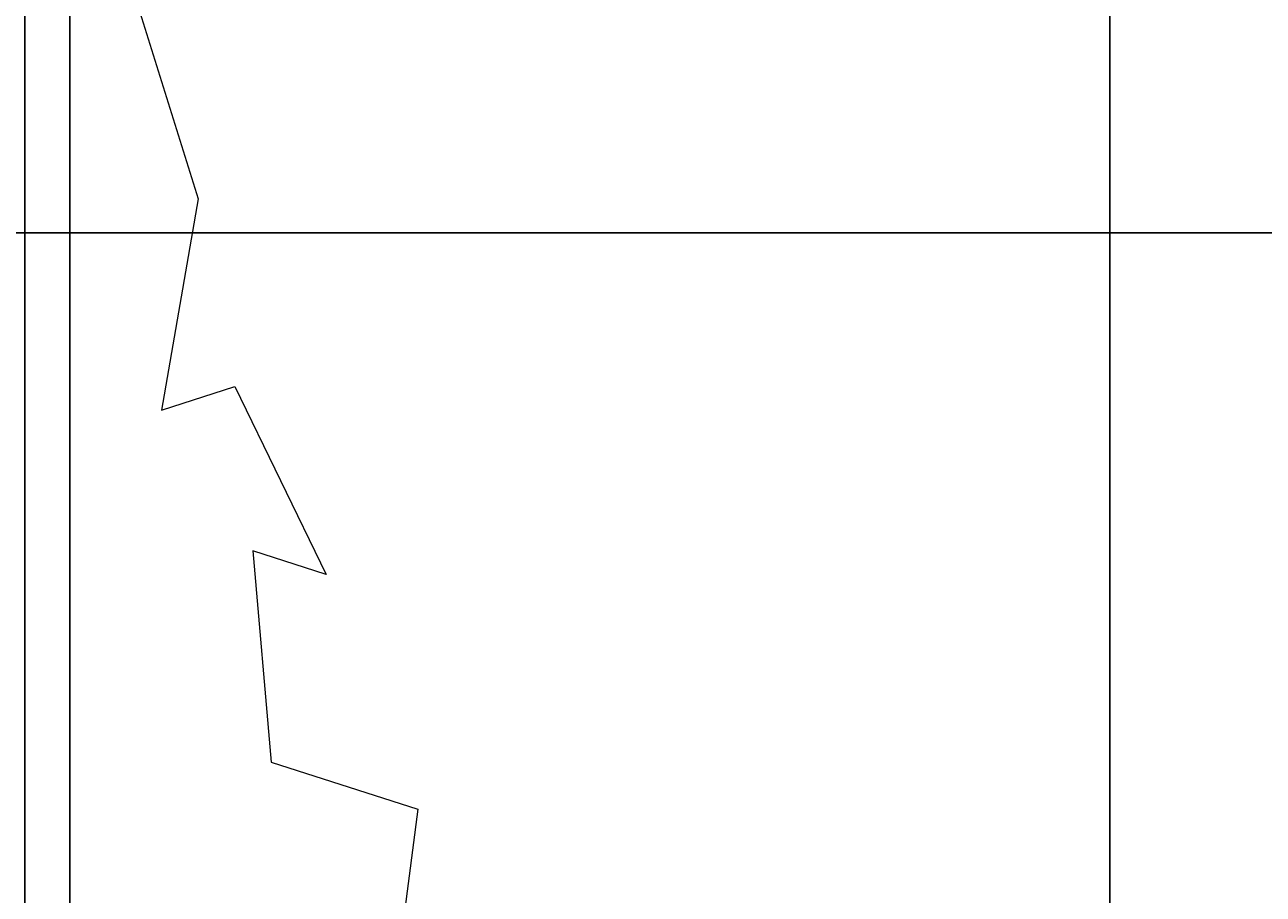
# Model space of a CAD drawing. Units: inches. Extents: x -26 to 776, y -22 to 650.
# Tile 46 of 62: x 426 to 506, y 102 to 158. Entities that reach past the tile are written whole.
import ezdxf

# ---------------------------------------------------------------- set-up
doc = ezdxf.new("R2010")
doc.units = ezdxf.units.IN
doc.header["$MEASUREMENT"] = 0
doc.layers.add('A-ANNO-DIMS', color=2, linetype='Continuous', lineweight=18)
doc.layers.add('L-PLNT-TREE', color=94, linetype='Continuous', lineweight=18)
doc.styles.get("Standard").update_dxf_attribs({"font": 'arial.ttf'})
doc.dimstyles.get("Standard").update_dxf_attribs({"dimtxt": 0.5625, "dimasz": 0.18, "dimexe": 0.18, "dimexo": 0.0625, "dimgap": 0.09, "dimtad": 0, "dimtih": 1, "dimtoh": 1, "dimdec": 4, "dimzin": 0, "dimdsep": 46, "dimlunit": 4, "dimtxsty": 'Standard', "dimcen": 0.09, "dimadec": 0, "dimazin": 0, "dimtfac": 1, "dimtdec": 4, "dimtofl": 0, "dimtmove": 0, "dimatfit": 3, "dimfxl": 1, "dimtolj": 1, "dimtzin": 0, "dimarcsym": 0})

# ---------------------------------------------------------------- blocks, each defined once
blk = doc.blocks.new('Tree - type 2 deciduous elevation')
blk.add_lwpolyline([(-34.386, 107.646), (-40.712, 98.798), (-37.261, 95.849), (-40.712, 90.688), (-41.287, 80.366), (-38.412, 78.154), (-36.686, 70.781), (-39.562, 71.518), (-37.261, 64.145), (-38.412, 57.509), (-36.111, 58.247), (-33.236, 52.348), (-35.536, 53.086), (-34.961, 46.45), (-30.36, 44.975), (-31.51, 36.128)])
blk = doc.blocks.new('*D20')
at = {"layer": 'A-ANNO-DIMS', "color": 0, "lineweight": -2, "transparency": 16777216}
for p, q in [((425.806, 455.472), (775.335, 455.472)), ((775.155, 455.292), (775.155, 235.854)), ((775.155, 15.662), (775.155, 235.1)), ((425.806, 15.482), (775.335, 15.482))]:
    blk.add_line(p, q, dxfattribs=at)
at = {"layer": 'A-ANNO-DIMS', "color": 0, "transparency": 16777216}
for points in [[(775.125, 455.292), (775.185, 455.292), (775.155, 455.472)], [(775.125, 15.662), (775.185, 15.662), (775.155, 15.482)]]:
    blk.add_solid(points, dxfattribs=at)
at = {"layer": 'Defpoints', "color": 0, "transparency": 16777216}
for p in [(425.743, 455.472), (775.155, 455.472), (425.743, 15.482)]:
    blk.add_point(p, dxfattribs=at)
at = {"layer": 'A-ANNO-DIMS', "color": 0, "transparency": 16777216, "insert": (775.155, 235.477), "char_height": 0.5625, "attachment_point": 5}
blk.add_mtext('\\A1;440', dxfattribs=at)
blk = doc.blocks.new('*D30')
at = {"layer": 'A-ANNO-DIMS', "color": 0, "lineweight": -2, "transparency": 16777216}
for p, q in [((280.68, 144.836), (775.335, 144.836)), ((775.155, 144.656), (775.155, 86.007)), ((775.155, 26.604), (775.155, 85.253)), ((280.68, 26.424), (775.335, 26.424))]:
    blk.add_line(p, q, dxfattribs=at)
at = {"layer": 'A-ANNO-DIMS', "color": 0, "transparency": 16777216}
for points in [[(775.125, 144.656), (775.185, 144.656), (775.155, 144.836)], [(775.125, 26.604), (775.185, 26.604), (775.155, 26.424)]]:
    blk.add_solid(points, dxfattribs=at)
at = {"layer": 'Defpoints', "color": 0, "transparency": 16777216}
for p in [(280.617, 144.836), (775.155, 144.836), (280.617, 26.424)]:
    blk.add_point(p, dxfattribs=at)
at = {"layer": 'A-ANNO-DIMS', "color": 0, "transparency": 16777216, "insert": (775.155, 85.63), "char_height": 0.5625, "attachment_point": 5}
blk.add_mtext('\\A1;118.41', dxfattribs=at)
blk = doc.blocks.new('*D39')
at = {"layer": 'A-ANNO-DIMS', "color": 0, "lineweight": -2, "transparency": 16777216}
for p, q in [((289.242, 15.545), (289.242, 649.856)), ((289.422, 649.676), (356.478, 649.676)), ((425.563, 649.676), (358.508, 649.676)), ((425.743, 15.545), (425.743, 649.856))]:
    blk.add_line(p, q, dxfattribs=at)
at = {"layer": 'A-ANNO-DIMS', "color": 0, "transparency": 16777216}
for points in [[(289.422, 649.706), (289.422, 649.646), (289.242, 649.676)], [(425.563, 649.706), (425.563, 649.646), (425.743, 649.676)]]:
    blk.add_solid(points, dxfattribs=at)
at = {"layer": 'Defpoints', "color": 0, "transparency": 16777216}
for p in [(425.743, 649.676), (289.242, 15.482), (425.743, 15.482)]:
    blk.add_point(p, dxfattribs=at)
at = {"layer": 'A-ANNO-DIMS', "color": 0, "transparency": 16777216, "insert": (357.493, 649.676), "char_height": 0.5625, "attachment_point": 5}
blk.add_mtext('\\A1;136.5', dxfattribs=at)
blk = doc.blocks.new('*D40')
at = {"layer": 'A-ANNO-DIMS', "color": 0, "lineweight": -2, "transparency": 16777216}
for p, q in [((425.743, 15.545), (425.743, 649.856)), ((425.923, 649.676), (459.646, 649.676)), ((495.451, 649.676), (461.728, 649.676)), ((495.631, 15.545), (495.631, 649.856))]:
    blk.add_line(p, q, dxfattribs=at)
at = {"layer": 'A-ANNO-DIMS', "color": 0, "transparency": 16777216}
for points in [[(425.923, 649.706), (425.923, 649.646), (425.743, 649.676)], [(495.451, 649.706), (495.451, 649.646), (495.631, 649.676)]]:
    blk.add_solid(points, dxfattribs=at)
at = {"layer": 'Defpoints', "color": 0, "transparency": 16777216}
for p in [(495.631, 649.676), (425.743, 15.482), (495.631, 15.482)]:
    blk.add_point(p, dxfattribs=at)
at = {"layer": 'A-ANNO-DIMS', "color": 0, "transparency": 16777216, "insert": (460.687, 649.676), "char_height": 0.5625, "attachment_point": 5}
blk.add_mtext('\\A1;69.89', dxfattribs=at)
blk = doc.blocks.new('*D47')
at = {"layer": 'A-ANNO-DIMS', "color": 0, "lineweight": -2, "transparency": 16777216}
for p, q in [((584.343, 199.901), (584.343, -21.315)), ((428.648, 180.243), (428.648, -21.315)), ((428.828, -21.135), (505.483, -21.135)), ((584.163, -21.135), (507.508, -21.135))]:
    blk.add_line(p, q, dxfattribs=at)
at = {"layer": 'A-ANNO-DIMS', "color": 0, "transparency": 16777216}
for points in [[(428.828, -21.105), (428.828, -21.165), (428.648, -21.135)], [(584.163, -21.105), (584.163, -21.165), (584.343, -21.135)]]:
    blk.add_solid(points, dxfattribs=at)
at = {"layer": 'Defpoints', "color": 0, "transparency": 16777216}
for p in [(584.343, 199.963), (428.648, 180.305), (584.343, -21.135)]:
    blk.add_point(p, dxfattribs=at)
at = {"layer": 'A-ANNO-DIMS', "color": 0, "transparency": 16777216, "insert": (506.496, -21.135), "char_height": 0.5625, "attachment_point": 5}
blk.add_mtext('\\A1;155.7', dxfattribs=at)

msp = doc.modelspace()

# ---------------------------------------------------------------- block references
at = {"layer": 'L-PLNT-TREE', "xscale": 2.050905272406618, "yscale": 2.050905272406618, "zscale": 2.050905272406618}
msp.add_blockref('Tree - type 2 deciduous elevation', (513.3241, 15.4824), dxfattribs=at)

# ---------------------------------------------------------------- dimensions: what is measured, and where the dimension line sits
at = {"layer": 'A-ANNO-DIMS'}
for base, p1, p2, override, picture, middle in [((425.7434, 649.6763), (289.2424, 15.4824), (425.7434, 15.4824), {"dimdec": 1, "dimlfac": 1, "dimrnd": 0, "dimzin": 0, "dimdsep": 46, "dimlunit": 2}, '*D39', (357.4929, 649.6763)), ((495.6309, 649.6763), (425.7434, 15.4824), (495.6309, 15.4824), {"dimdec": 2, "dimlfac": 1, "dimrnd": 0, "dimzin": 0, "dimdsep": 46, "dimlunit": 2}, '*D40', (460.6872, 649.6763)), ((584.3428, -21.1349), (428.6484, 180.3054), (584.3428, 199.9634), {"dimdec": 1, "dimlfac": 1, "dimrnd": 0, "dimzin": 0, "dimdsep": 46, "dimlunit": 2}, '*D47', (506.4956, -21.1349))]:
    dim = msp.add_linear_dim(base=base, p1=p1, p2=p2, dimstyle='Standard', override=override, dxfattribs=at)
    dim.commit()
    dim.dimension.update_dxf_attribs({"geometry": picture, "text_midpoint": middle})
for base, p1, p2, override, picture, middle in [((775.1553, 455.4717), (425.7434, 15.4824), (425.7434, 455.4717), {"dimdec": 0, "dimlfac": 1, "dimrnd": 0, "dimzin": 0, "dimdsep": 46, "dimlunit": 2}, '*D20', (775.1553, 235.477)), ((775.1553, 144.8359), (280.6173, 26.4239), (280.6173, 144.8359), {"dimdec": 2, "dimlfac": 1, "dimrnd": 0, "dimzin": 0, "dimdsep": 46, "dimlunit": 2}, '*D30', (775.1553, 85.6299))]:
    dim = msp.add_linear_dim(base=base, p1=p1, p2=p2, angle=90, dimstyle='Standard', override=override, dxfattribs=at)
    dim.commit()
    dim.dimension.update_dxf_attribs({"geometry": picture, "text_midpoint": middle})

doc.saveas('drawing.dxf')
